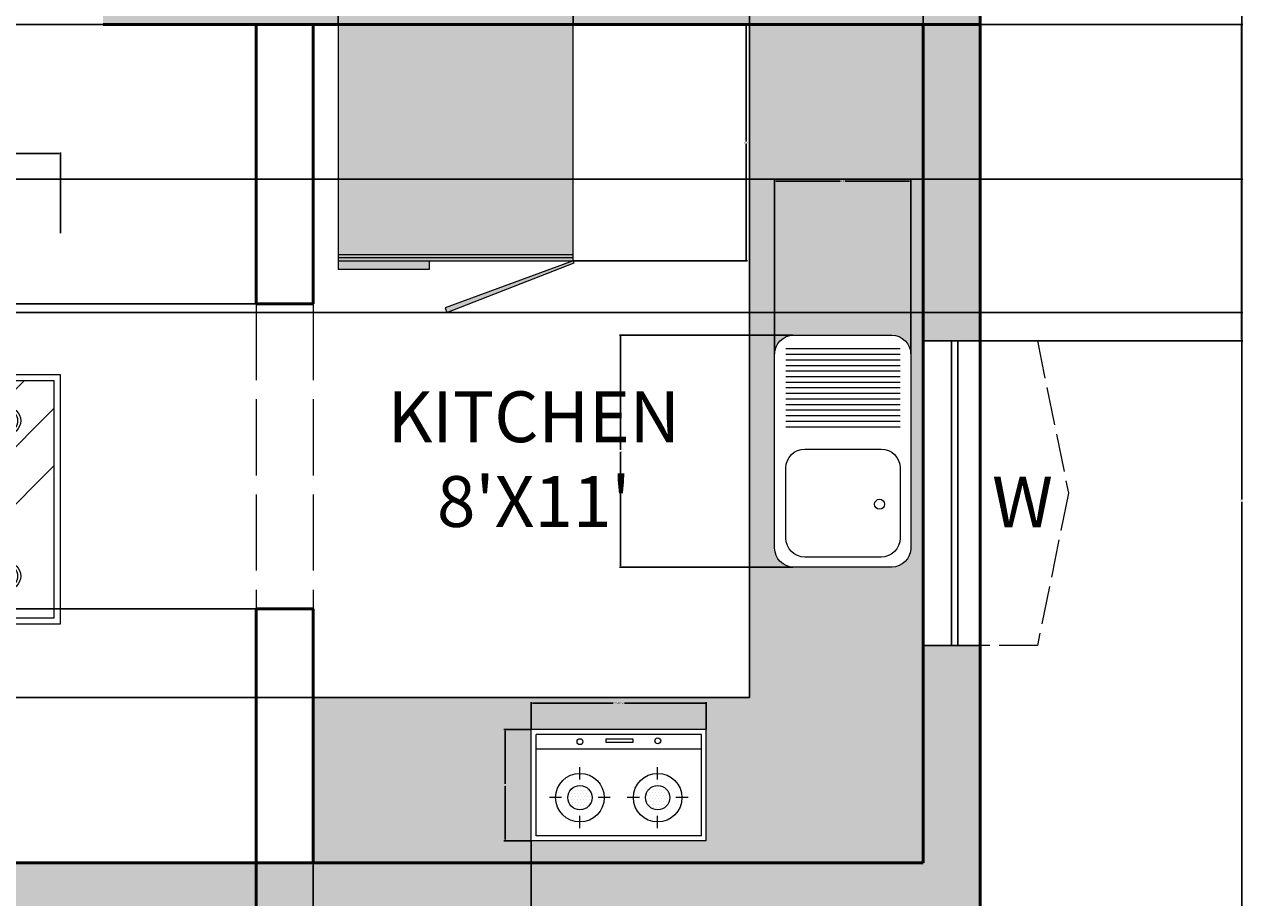
# Model space of a CAD drawing. Units: inches. Extents: x -75 to 416, y -487 to 70.
# Tile 4 of 5: x 224 to 416, y -271 to -133. Entities that reach past the tile are written whole.
import ezdxf

# ---------------------------------------------------------------- set-up
doc = ezdxf.new("R2010")
doc.units = ezdxf.units.IN
doc.header["$MEASUREMENT"] = 0
doc.linetypes.add('ACAD_ISO02W100', pattern=[15, 12, -3])
for name, color, linetype, lineweight in [('A-ANNO-DIMS', 2, 'Continuous', 18), ('A-ANNO-TEXT', 7, 'Continuous', 18), ('A-AREA-IDEN', 7, 'Continuous', 25), ('A-EQPM', 8, 'Continuous', 18), ('A-EQPM-PATT', 252, 'Continuous', 13), ('A-FLOR-CASE', 8, 'Continuous', 25), ('A-FLOR-CASE-PATT', 252, 'Continuous', 13), ('A-FLOR-FIXT', 9, 'Continuous', 18), ('A-FLOR-FIXT-PATT', 9, 'Continuous', 13), ('A-FURN', 8, 'Continuous', 18), ('A-GLAZ', 4, 'Continuous', 25), ('A-GLAZ-OVHD', 4, 'ACAD_ISO02W100', 13), ('A-WALL', 7, 'Continuous', 50), ('A-WALL-OVHD', 7, 'ACAD_ISO02W100', 18), ('A-WALL-PATT', 252, 'Continuous', 13)]:
    doc.layers.add(name, color=color, linetype=linetype, lineweight=lineweight)
doc.styles.get("Standard").update_dxf_attribs({"font": 'arial.ttf'})
doc.dimstyles.get("Standard").update_dxf_attribs({"dimtxt": 0.18, "dimasz": 0.18, "dimexe": 0.18, "dimexo": 0.0625, "dimgap": 0.09, "dimtad": 0, "dimtih": 1, "dimtoh": 1, "dimdec": 4, "dimzin": 0, "dimdsep": 46, "dimtxsty": 'Standard', "dimcen": 0.09, "dimadec": 0, "dimazin": 0, "dimtfac": 1, "dimtdec": 4, "dimtofl": 0, "dimtmove": 0, "dimatfit": 3, "dimfxl": 1, "dimtolj": 1, "dimtzin": 0, "dimarcsym": 0})

# ---------------------------------------------------------------- blocks, each defined once
blk = doc.blocks.new('A$C0FD55737')
for p, q in [((0.2013, 1.6134), (0.1562, 1.3384)), ((0.4912, 1.6302), (0.2211, 1.6302)), ((0.511, 1.6134), (0.5562, 1.3384)), ((0.8828, 1.6134), (0.8376, 1.3384)), ((0.9026, 1.6302), (1.1727, 1.6302)), ((1.1925, 1.6134), (1.2376, 1.3384)), ((0.2362, 1.2584), (0.4762, 1.2584)), ((1.1576, 1.2584), (0.9176, 1.2584)), ((0, 1.2513), (0, 0.4513)), ((1.4, 1.2513), (0, 1.2513)), ((0.02, 1.0725), (0.1788, 1.2313)), ((0.02, 0.7043), (0.547, 1.2313)), ((1.38, 1.2313), (0.02, 1.2313)), ((0.02, 1.2313), (0.02, 0.4713)), ((0.2189, 1.0873), (0.3629, 1.2313)), ((0.3393, 0.4713), (1.0993, 1.2313)), ((0.5234, 0.4713), (1.2834, 1.2313)), ((1.38, 0.4713), (1.38, 1.2313)), ((1.4, 0.4513), (1.4, 1.2513)), ((0.7074, 0.4713), (1.38, 1.1438)), ((0.02, 0.8884), (0.1931, 1.0614)), ((0.8915, 0.4713), (1.38, 0.9597)), ((0.02, 0.4713), (1.38, 0.4713)), ((0, 0.4513), (1.4, 0.4513)), ((0.2362, 0.4371), (0.4762, 0.4371)), ((1.1576, 0.4371), (0.9176, 0.4371)), ((0.2013, 0.0821), (0.1562, 0.3571)), ((0.511, 0.0821), (0.5562, 0.3571)), ((0.8828, 0.0821), (0.8376, 0.3571)), ((1.1925, 0.0821), (1.2376, 0.3571)), ((0.4912, 0.0653), (0.2211, 0.0653)), ((0.9026, 0.0653), (1.1727, 0.0653))]:
    blk.add_line(p, q)
for centre, radius in [((0.1766, 1.1037), 0.0454), ((0.1766, 1.1037), 0.0354), ((1.227, 1.1037), 0.0454), ((1.227, 1.1037), 0.0354), ((0.1766, 0.6052), 0.0454), ((0.1766, 0.6052), 0.0354), ((1.227, 0.6052), 0.0454), ((1.227, 0.6052), 0.0354)]:
    blk.add_circle(centre, radius)
for centre, radius, start, end in [((0.3562, 0.9712), 0.7243, 74.4701, 105.577), ((1.0376, 0.9712), 0.7243, 74.423, 105.5299), ((0.1662, 1.6546), 0.015, 105.4901, 284.2842), ((0.3562, 0.9716), 0.6939, 74.4325, 105.5675), ((0.5461, 1.6546), 0.015, 255.7158, 74.5099), ((0.8477, 1.6546), 0.015, 105.4901, 284.2842), ((1.0376, 0.9716), 0.6939, 74.4325, 105.5675), ((1.2276, 1.6546), 0.015, 255.7158, 74.5099), ((0.2211, 1.6102), 0.02, 90, 170.6717), ((0.4912, 1.6102), 0.02, 9.3283, 90), ((0.9026, 1.6102), 0.02, 90, 170.6717), ((1.1727, 1.6102), 0.02, 9.3283, 90), ((0.2362, 1.3384), 0.08, 180, 270), ((0.4762, 1.3384), 0.08, 270, 0), ((0.9176, 1.3384), 0.08, 180, 270), ((1.1576, 1.3384), 0.08, 270, 0), ((0.2362, 0.3571), 0.08, 90, 180), ((0.4762, 0.3571), 0.08, 0, 90), ((0.9176, 0.3571), 0.08, 90, 180), ((1.1576, 0.3571), 0.08, 0, 90), ((0.2211, 0.0853), 0.02, 189.3283, 270), ((0.4912, 0.0853), 0.02, 270, 350.6717), ((0.9026, 0.0853), 0.02, 189.3283, 270), ((1.1727, 0.0853), 0.02, 270, 350.6717), ((0.1662, 0.0409), 0.015, 75.7158, 254.5099), ((0.3562, 0.7239), 0.6939, 254.4325, 285.5675), ((0.5461, 0.0409), 0.015, 285.4901, 104.2842), ((0.8477, 0.0409), 0.015, 75.7158, 254.5099), ((1.0376, 0.7239), 0.6939, 254.4325, 285.5675), ((1.2276, 0.0409), 0.015, 285.4901, 104.2842), ((0.3562, 0.7243), 0.7243, 254.423, 285.5299), ((1.0376, 0.7243), 0.7243, 254.4701, 285.577)]:
    blk.add_arc(centre, radius, start, end)
blk = doc.blocks.new('A$C475E21CF')
for p, q in [((0, 444.5), (0, 0)), ((0, 444.5), (699.9, 444.5)), ((699.9, 444.5), (699.9, 0)), ((19.4, 425), (19.4, 19.4)), ((19.4, 425), (680.5, 425)), ((194.5, 393.9), (194.5, 345.2)), ((505.4, 393.9), (505.4, 345.2)), ((680.5, 425), (680.5, 19.4)), ((166.9, 300.5), (166.9, 300.5)), ((179.1, 300.5), (179.1, 300.5)), ((185.2, 312.7), (185.2, 312.7)), ((191.2, 300.5), (191.2, 300.5)), ((197.3, 312.7), (197.3, 312.7)), ((203.4, 300.5), (203.4, 300.5)), ((209.5, 312.7), (209.5, 312.7)), ((215.6, 300.5), (215.6, 300.5)), ((227.7, 300.5), (227.7, 300.5)), ((480.2, 304.5), (480.2, 304.5)), ((492.3, 304.5), (492.3, 304.5)), ((498.4, 316.6), (498.4, 316.6)), ((504.5, 304.5), (504.5, 304.5)), ((510.6, 316.6), (510.6, 316.6)), ((516.7, 304.5), (516.7, 304.5)), ((522.7, 316.6), (522.7, 316.6)), ((528.8, 304.5), (528.8, 304.5)), ((541, 304.5), (541, 304.5)), ((72.9, 272.3), (121.6, 272.3)), ((148.7, 264.1), (148.7, 264.1)), ((154.8, 276.2), (154.8, 276.2)), ((154.8, 251.9), (154.8, 251.9)), ((160.9, 288.4), (160.9, 288.4)), ((160.9, 264.1), (160.9, 264.1)), ((166.9, 276.2), (166.9, 276.2)), ((166.9, 251.9), (166.9, 251.9)), ((173, 288.4), (173, 288.4)), ((173, 264.1), (173, 264.1)), ((179.1, 276.2), (179.1, 276.2)), ((179.1, 251.9), (179.1, 251.9)), ((185.2, 288.4), (185.2, 288.4)), ((185.2, 264.1), (185.2, 264.1)), ((191.2, 276.2), (191.2, 276.2)), ((191.2, 251.9), (191.2, 251.9)), ((197.3, 288.4), (197.3, 288.4)), ((197.3, 264.1), (197.3, 264.1)), ((203.4, 276.2), (203.4, 276.2)), ((203.4, 251.9), (203.4, 251.9)), ((209.5, 288.4), (209.5, 288.4)), ((209.5, 264.1), (209.5, 264.1)), ((215.6, 276.2), (215.6, 276.2)), ((215.6, 251.9), (215.6, 251.9)), ((221.6, 288.4), (221.6, 288.4)), ((221.6, 264.1), (221.6, 264.1)), ((227.7, 276.2), (227.7, 276.2)), ((227.7, 251.9), (227.7, 251.9)), ((233.8, 288.4), (233.8, 288.4)), ((233.8, 264.1), (233.8, 264.1)), ((239.9, 276.2), (239.9, 276.2)), ((239.9, 251.9), (239.9, 251.9)), ((267.4, 272.3), (316, 272.3)), ((383.9, 272.3), (432.5, 272.3)), ((462, 268), (462, 268)), ((468, 280.2), (468, 280.2)), ((468, 255.9), (468, 255.9)), ((474.1, 292.3), (474.1, 292.3)), ((474.1, 268), (474.1, 268)), ((480.2, 280.2), (480.2, 280.2)), ((480.2, 255.9), (480.2, 255.9)), ((486.3, 292.3), (486.3, 292.3)), ((486.3, 268), (486.3, 268)), ((492.3, 280.2), (492.3, 280.2)), ((492.3, 255.9), (492.3, 255.9)), ((498.4, 292.3), (498.4, 292.3)), ((498.4, 268), (498.4, 268)), ((504.5, 280.2), (504.5, 280.2)), ((504.5, 255.9), (504.5, 255.9)), ((510.6, 292.3), (510.6, 292.3)), ((510.6, 268), (510.6, 268)), ((516.7, 280.2), (516.7, 280.2)), ((516.7, 255.9), (516.7, 255.9)), ((522.7, 292.3), (522.7, 292.3)), ((522.7, 268), (522.7, 268)), ((528.8, 280.2), (528.8, 280.2)), ((528.8, 255.9), (528.8, 255.9)), ((534.9, 292.3), (534.9, 292.3)), ((534.9, 268), (534.9, 268)), ((541, 280.2), (541, 280.2)), ((541, 255.9), (541, 255.9)), ((547, 292.3), (547, 292.3)), ((547, 268), (547, 268)), ((553.1, 280.2), (553.1, 280.2)), ((553.1, 255.9), (553.1, 255.9)), ((578.4, 272.3), (627, 272.3)), ((160.9, 239.8), (160.9, 239.8)), ((173, 239.8), (173, 239.8)), ((179.1, 227.6), (179.1, 227.6)), ((185.2, 239.8), (185.2, 239.8)), ((191.2, 227.6), (191.2, 227.6)), ((194.5, 199.4), (194.5, 150.8)), ((197.3, 239.8), (197.3, 239.8)), ((203.4, 227.6), (203.4, 227.6)), ((209.5, 239.8), (209.5, 239.8)), ((215.6, 227.6), (215.6, 227.6)), ((221.6, 239.8), (221.6, 239.8)), ((233.8, 239.8), (233.8, 239.8)), ((474.1, 243.7), (474.1, 243.7)), ((486.3, 243.7), (486.3, 243.7)), ((492.3, 231.5), (492.3, 231.5)), ((498.4, 243.7), (498.4, 243.7)), ((504.5, 231.5), (504.5, 231.5)), ((505.4, 199.4), (505.4, 150.8)), ((510.6, 243.7), (510.6, 243.7)), ((516.7, 231.5), (516.7, 231.5)), ((522.7, 243.7), (522.7, 243.7)), ((528.8, 231.5), (528.8, 231.5)), ((534.9, 243.7), (534.9, 243.7)), ((547, 243.7), (547, 243.7)), ((19.4, 77.8), (680.5, 77.8)), ((293.4, 51.9), (400.6, 51.9)), ((293.4, 36.5), (293.4, 51.9)), ((400.6, 51.9), (400.6, 36.5)), ((0, 0), (699.9, 0)), ((19.4, 19.4), (680.5, 19.4)), ((400.6, 36.5), (293.4, 36.5))]:
    blk.add_line(p, q)
for centre, radius in [((194.5, 272.3), 97.2), ((505.4, 272.3), 97.2), ((194.5, 272.3), 48.6), ((505.4, 272.3), 48.6), ((193.9, 45.1), 11.7), ((505.2, 48.5), 11.7)]:
    blk.add_circle(centre, radius)
blk = doc.blocks.new('WIN-48IN')
for p, q in [((0, 9), (0, 0)), ((48, 9), (48, 0)), ((48, 5.5), (0, 5.5)), ((48, 4.5), (0, 4.5))]:
    blk.add_line(p, q)
blk = doc.blocks.new('WIN-SHADE-48IN')
at = {"ltscale": 0.5}
for p, q in [((0, 4.91), (0, 13.91)), ((48, 13.91), (48, 4.91)), ((24, 0), (0, 4.91)), ((48, 4.91), (24, 0))]:
    blk.add_line(p, q, dxfattribs=at)
blk = doc.blocks.new('*D29')
at = {"layer": 'A-ANNO-DIMS', "color": 0, "lineweight": -2, "transparency": 16777216}
for p, q in [((161.08, -166.25), (161.08, -153.53)), ((229.74, -166.25), (229.74, -153.53)), ((161.26, -153.71), (195.2, -153.71)), ((229.56, -153.71), (195.63, -153.71))]:
    blk.add_line(p, q, dxfattribs=at)
at = {"layer": 'A-ANNO-DIMS', "color": 0, "transparency": 16777216}
for points in [[(161.26, -153.68), (161.26, -153.74), (161.08, -153.71)], [(229.56, -153.68), (229.56, -153.74), (229.74, -153.71)]]:
    blk.add_solid(points, dxfattribs=at)
at = {"layer": 'Defpoints', "color": 0, "transparency": 16777216}
for p in [(229.74, -153.71), (161.08, -166.31), (229.74, -166.31)]:
    blk.add_point(p, dxfattribs=at)
at = {"layer": 'A-ANNO-DIMS', "color": 0, "transparency": 16777216, "insert": (195.41, -153.71), "char_height": 0.18, "attachment_point": 5}
blk.add_mtext('\\A1;69', dxfattribs=at)
blk = doc.blocks.new('*D30')
at = {"layer": 'A-ANNO-DIMS', "color": 0, "lineweight": -2, "transparency": 16777216}
for p, q in [((303.87, -244.32), (303.87, -240.07)), ((304.05, -240.25), (316.77, -240.25)), ((331.25, -240.25), (318.53, -240.25)), ((331.43, -244.32), (331.43, -240.07))]:
    blk.add_line(p, q, dxfattribs=at)
at = {"layer": 'A-ANNO-DIMS', "color": 0, "transparency": 16777216}
for points in [[(304.05, -240.22), (304.05, -240.28), (303.87, -240.25)], [(331.25, -240.22), (331.25, -240.28), (331.43, -240.25)]]:
    blk.add_solid(points, dxfattribs=at)
at = {"layer": 'Defpoints', "color": 0, "transparency": 16777216}
for p in [(303.87, -240.25), (303.87, -244.38), (331.43, -244.38)]:
    blk.add_point(p, dxfattribs=at)
at = {"layer": 'A-ANNO-DIMS', "color": 0, "transparency": 16777216, "insert": (317.65, -240.25), "char_height": 0.18, "attachment_point": 5}
blk.add_mtext('\\A1;COOKTOP 28', dxfattribs=at)
blk = doc.blocks.new('*D31')
at = {"layer": 'A-ANNO-DIMS', "color": 0, "lineweight": -2, "transparency": 16777216}
for p, q in [((303.81, -244.38), (299.56, -244.38)), ((299.74, -244.56), (299.74, -252.95)), ((299.74, -261.7), (299.74, -253.31)), ((303.81, -261.88), (299.56, -261.88))]:
    blk.add_line(p, q, dxfattribs=at)
at = {"layer": 'A-ANNO-DIMS', "color": 0, "transparency": 16777216}
for points in [[(299.71, -244.56), (299.77, -244.56), (299.74, -244.38)], [(299.71, -261.7), (299.77, -261.7), (299.74, -261.88)]]:
    blk.add_solid(points, dxfattribs=at)
at = {"layer": 'Defpoints', "color": 0, "transparency": 16777216}
for p in [(303.87, -244.38), (299.74, -261.88), (303.87, -261.88)]:
    blk.add_point(p, dxfattribs=at)
at = {"layer": 'A-ANNO-DIMS', "color": 0, "transparency": 16777216, "insert": (299.74, -253.13), "char_height": 0.18, "attachment_point": 5}
blk.add_mtext('\\A1;17', dxfattribs=at)
blk = doc.blocks.new('*D35')
at = {"layer": 'A-ANNO-DIMS', "color": 0, "lineweight": -2, "transparency": 16777216}
for p, q in [((374.615553, 28.625508), (415.902741, 28.625508)), ((415.722741, 28.445508), (415.722741, -208.194492)), ((415.722741, -445.194492), (415.722741, -208.554492)), ((374.615553, -445.374492), (415.902741, -445.374492))]:
    blk.add_line(p, q, dxfattribs=at)
at = {"layer": 'A-ANNO-DIMS', "color": 0, "transparency": 16777216}
for points in [[(415.692741, 28.445508), (415.752741, 28.445508), (415.722741, 28.625508)], [(415.692741, -445.194492), (415.752741, -445.194492), (415.722741, -445.374492)]]:
    blk.add_solid(points, dxfattribs=at)
at = {"layer": 'Defpoints', "color": 0, "transparency": 16777216}
for p in [(374.553053, 28.625508), (374.553053, -445.374492), (415.722741, -445.374492)]:
    blk.add_point(p, dxfattribs=at)
at = {"layer": 'A-ANNO-DIMS', "color": 0, "transparency": 16777216, "insert": (415.722741, -208.374492), "char_height": 0.18, "attachment_point": 5}
blk.add_mtext('\\A1;474', dxfattribs=at)
blk = doc.blocks.new('*D41')
at = {"layer": 'A-ANNO-DIMS', "color": 0, "lineweight": -2, "transparency": 16777216}
for p, q in [((374.62, -133.37), (415.9, -133.37)), ((415.72, -133.55), (415.72, -158.09)), ((415.72, -182.99), (415.72, -158.45)), ((374.62, -183.17), (415.9, -183.17))]:
    blk.add_line(p, q, dxfattribs=at)
at = {"layer": 'A-ANNO-DIMS', "color": 0, "transparency": 16777216}
for points in [[(415.69, -133.55), (415.75, -133.55), (415.72, -133.37)], [(415.69, -182.99), (415.75, -182.99), (415.72, -183.17)]]:
    blk.add_solid(points, dxfattribs=at)
at = {"layer": 'Defpoints', "color": 0, "transparency": 16777216}
for p in [(374.55, -133.37), (374.55, -183.17), (415.72, -183.17)]:
    blk.add_point(p, dxfattribs=at)
at = {"layer": 'A-ANNO-DIMS', "color": 0, "transparency": 16777216, "insert": (415.72, -158.27), "char_height": 0.18, "attachment_point": 5}
blk.add_mtext('\\A1;49.79', dxfattribs=at)
blk = doc.blocks.new('*D52')
at = {"layer": 'A-ANNO-DIMS', "color": 0, "lineweight": -2, "transparency": 16777216}
for p, q in [((260.49, -133.37), (-74.89, -133.37)), ((-74.71, -133.55), (-74.71, -155.19)), ((-74.71, -177.19), (-74.71, -155.55)), ((260.49, -177.37), (-74.89, -177.37))]:
    blk.add_line(p, q, dxfattribs=at)
at = {"layer": 'A-ANNO-DIMS', "color": 0, "transparency": 16777216}
for points in [[(-74.74, -133.55), (-74.68, -133.55), (-74.71, -133.37)], [(-74.74, -177.19), (-74.68, -177.19), (-74.71, -177.37)]]:
    blk.add_solid(points, dxfattribs=at)
at = {"layer": 'Defpoints', "color": 0, "transparency": 16777216}
for p in [(260.55, -133.37), (-74.71, -177.37), (260.55, -177.37)]:
    blk.add_point(p, dxfattribs=at)
at = {"layer": 'A-ANNO-DIMS', "color": 0, "transparency": 16777216, "insert": (-74.71, -155.37), "char_height": 0.18, "attachment_point": 5}
blk.add_mtext('\\A1;43.99', dxfattribs=at)
blk = doc.blocks.new('*D53')
at = {"layer": 'A-ANNO-DIMS', "color": 0, "lineweight": -2, "transparency": 16777216}
for p, q in [((260.49, -177.37), (-74.89, -177.37)), ((-74.71, -177.55), (-74.71, -201.19)), ((-74.71, -225.19), (-74.71, -201.55)), ((260.49, -225.37), (-74.89, -225.37))]:
    blk.add_line(p, q, dxfattribs=at)
at = {"layer": 'A-ANNO-DIMS', "color": 0, "transparency": 16777216}
for points in [[(-74.74, -177.55), (-74.68, -177.55), (-74.71, -177.37)], [(-74.74, -225.19), (-74.68, -225.19), (-74.71, -225.37)]]:
    blk.add_solid(points, dxfattribs=at)
at = {"layer": 'Defpoints', "color": 0, "transparency": 16777216}
for p in [(260.55, -177.37), (-74.71, -225.37), (260.55, -225.37)]:
    blk.add_point(p, dxfattribs=at)
at = {"layer": 'A-ANNO-DIMS', "color": 0, "transparency": 16777216, "insert": (-74.71, -201.37), "char_height": 0.18, "attachment_point": 5}
blk.add_mtext('\\A1;48', dxfattribs=at)
blk = doc.blocks.new('*D54')
at = {"layer": 'A-ANNO-DIMS', "color": 0, "lineweight": -2, "transparency": 16777216}
for p, q in [((338.22, -133.31), (338.22, 69.98)), ((338.4, 69.8), (351.49, 69.8)), ((365.37, 69.8), (352.28, 69.8)), ((365.55, -133.31), (365.55, 69.98))]:
    blk.add_line(p, q, dxfattribs=at)
at = {"layer": 'A-ANNO-DIMS', "color": 0, "transparency": 16777216}
for points in [[(338.4, 69.83), (338.4, 69.77), (338.22, 69.8)], [(365.37, 69.83), (365.37, 69.77), (365.55, 69.8)]]:
    blk.add_solid(points, dxfattribs=at)
at = {"layer": 'Defpoints', "color": 0, "transparency": 16777216}
for p in [(365.55, 69.8), (338.22, -133.37), (365.55, -133.37)]:
    blk.add_point(p, dxfattribs=at)
at = {"layer": 'A-ANNO-DIMS', "color": 0, "transparency": 16777216, "insert": (351.89, 69.8), "char_height": 0.18, "attachment_point": 5}
blk.add_mtext('\\A1;27.33', dxfattribs=at)
blk = doc.blocks.new('*D55')
at = {"layer": 'A-ANNO-DIMS', "color": 0, "lineweight": -2, "transparency": 16777216}
for p, q in [((269.49, -239.36), (-74.89, -239.36)), ((-74.71, -239.54), (-74.71, -252.19)), ((-74.71, -265.19), (-74.71, -252.55)), ((269.49, -265.37), (-74.89, -265.37))]:
    blk.add_line(p, q, dxfattribs=at)
at = {"layer": 'A-ANNO-DIMS', "color": 0, "transparency": 16777216}
for points in [[(-74.74, -239.54), (-74.68, -239.54), (-74.71, -239.36)], [(-74.74, -265.19), (-74.68, -265.19), (-74.71, -265.37)]]:
    blk.add_solid(points, dxfattribs=at)
at = {"layer": 'Defpoints', "color": 0, "transparency": 16777216}
for p in [(269.55, -239.36), (-74.71, -265.37), (269.55, -265.37)]:
    blk.add_point(p, dxfattribs=at)
at = {"layer": 'A-ANNO-DIMS', "color": 0, "transparency": 16777216, "insert": (-74.71, -252.37), "char_height": 0.18, "attachment_point": 5}
blk.add_mtext('\\A1;26.01', dxfattribs=at)
blk = doc.blocks.new('*D60')
at = {"layer": 'A-ANNO-DIMS', "color": 0, "lineweight": -2, "transparency": 16777216}
for p, q in [((12.62, -157.75), (415.9, -157.75)), ((415.72, -157.93), (415.72, -168.07)), ((415.72, -178.57), (415.72, -168.43)), ((12.62, -178.75), (415.9, -178.75))]:
    blk.add_line(p, q, dxfattribs=at)
at = {"layer": 'A-ANNO-DIMS', "color": 0, "transparency": 16777216}
for points in [[(415.69, -157.93), (415.75, -157.93), (415.72, -157.75)], [(415.69, -178.57), (415.75, -178.57), (415.72, -178.75)]]:
    blk.add_solid(points, dxfattribs=at)
at = {"layer": 'Defpoints', "color": 0, "transparency": 16777216}
for p in [(12.55, -157.75), (12.55, -178.75), (415.72, -178.75)]:
    blk.add_point(p, dxfattribs=at)
at = {"layer": 'A-ANNO-DIMS', "color": 0, "transparency": 16777216, "insert": (415.72, -168.25), "char_height": 0.18, "attachment_point": 5}
blk.add_mtext('\\A1;21', dxfattribs=at)
blk = doc.blocks.new('*D66')
at = {"layer": 'A-ANNO-DIMS', "color": 0, "lineweight": -2, "transparency": 16777216}
for p, q in [((273.46, -133.31), (273.46, 69.98)), ((273.64, 69.8), (291.5, 69.8)), ((310.28, 69.8), (292.43, 69.8)), ((310.46, -133.31), (310.46, 69.98))]:
    blk.add_line(p, q, dxfattribs=at)
at = {"layer": 'A-ANNO-DIMS', "color": 0, "transparency": 16777216}
for points in [[(273.64, 69.83), (273.64, 69.77), (273.46, 69.8)], [(310.28, 69.83), (310.28, 69.77), (310.46, 69.8)]]:
    blk.add_solid(points, dxfattribs=at)
at = {"layer": 'Defpoints', "color": 0, "transparency": 16777216}
for p in [(310.46, 69.8), (273.46, -133.37), (310.46, -133.37)]:
    blk.add_point(p, dxfattribs=at)
at = {"layer": 'A-ANNO-DIMS', "color": 0, "transparency": 16777216, "insert": (291.96, 69.8), "char_height": 0.18, "attachment_point": 5}
blk.add_mtext('\\A1;37.004', dxfattribs=at)
blk = doc.blocks.new('*D67')
at = {"layer": 'A-ANNO-DIMS', "color": 0, "lineweight": -2, "transparency": 16777216}
for p, q in [((310.53, -133.37), (337.9, -133.37)), ((337.72, -133.55), (337.72, -151.81)), ((337.72, -170.43), (337.72, -152.18)), ((310.53, -170.61), (337.9, -170.61))]:
    blk.add_line(p, q, dxfattribs=at)
at = {"layer": 'A-ANNO-DIMS', "color": 0, "transparency": 16777216}
for points in [[(337.69, -133.55), (337.75, -133.55), (337.72, -133.37)], [(337.69, -170.43), (337.75, -170.43), (337.72, -170.61)]]:
    blk.add_solid(points, dxfattribs=at)
at = {"layer": 'Defpoints', "color": 0, "transparency": 16777216}
for p in [(310.46, -133.37), (310.46, -170.61), (337.72, -170.61)]:
    blk.add_point(p, dxfattribs=at)
at = {"layer": 'A-ANNO-DIMS', "color": 0, "transparency": 16777216, "insert": (337.72, -151.99), "char_height": 0.18, "attachment_point": 5}
blk.add_mtext('\\A1;37.24', dxfattribs=at)
blk = doc.blocks.new('*D68')
at = {"layer": 'A-ANNO-DIMS', "color": 0, "lineweight": -2, "transparency": 16777216}
for p, q in [((345.13, -182.29), (317.75, -182.29)), ((317.93, -182.47), (317.93, -200.37)), ((317.93, -218.63), (317.93, -200.73)), ((345.13, -218.81), (317.75, -218.81))]:
    blk.add_line(p, q, dxfattribs=at)
at = {"layer": 'A-ANNO-DIMS', "color": 0, "transparency": 16777216}
for points in [[(317.9, -182.47), (317.96, -182.47), (317.93, -182.29)], [(317.9, -218.63), (317.96, -218.63), (317.93, -218.81)]]:
    blk.add_solid(points, dxfattribs=at)
at = {"layer": 'Defpoints', "color": 0, "transparency": 16777216}
for p in [(317.93, -182.29), (345.19, -182.29), (345.19, -218.81)]:
    blk.add_point(p, dxfattribs=at)
at = {"layer": 'A-ANNO-DIMS', "color": 0, "transparency": 16777216, "insert": (317.93, -200.55), "char_height": 0.18, "attachment_point": 5}
blk.add_mtext('\\A1;36.52', dxfattribs=at)
blk = doc.blocks.new('*D69')
at = {"layer": 'A-ANNO-DIMS', "color": 0, "lineweight": -2, "transparency": 16777216}
for p, q in [((342.19, -185.23), (342.19, -157.85)), ((342.37, -158.03), (352.51, -158.03)), ((363.44, -158.03), (353.3, -158.03)), ((363.62, -185.23), (363.62, -157.85))]:
    blk.add_line(p, q, dxfattribs=at)
at = {"layer": 'A-ANNO-DIMS', "color": 0, "transparency": 16777216}
for points in [[(342.37, -158), (342.37, -158.06), (342.19, -158.03)], [(363.44, -158), (363.44, -158.06), (363.62, -158.03)]]:
    blk.add_solid(points, dxfattribs=at)
at = {"layer": 'Defpoints', "color": 0, "transparency": 16777216}
for p in [(363.62, -158.03), (342.19, -185.29), (363.62, -185.29)]:
    blk.add_point(p, dxfattribs=at)
at = {"layer": 'A-ANNO-DIMS', "color": 0, "transparency": 16777216, "insert": (352.9, -158.03), "char_height": 0.18, "attachment_point": 5}
blk.add_mtext('\\A1;21.43', dxfattribs=at)
blk = doc.blocks.new('*D71')
at = {"layer": 'A-ANNO-DIMS', "color": 0, "lineweight": -2, "transparency": 16777216}
for p, q in [((303.87, -261.95), (303.87, -486.72)), ((269.55, -265.44), (269.55, -486.72)), ((269.73, -486.54), (286.32, -486.54)), ((303.69, -486.54), (287.11, -486.54))]:
    blk.add_line(p, q, dxfattribs=at)
at = {"layer": 'A-ANNO-DIMS', "color": 0, "transparency": 16777216}
for points in [[(269.73, -486.51), (269.73, -486.57), (269.55, -486.54)], [(303.69, -486.51), (303.69, -486.57), (303.87, -486.54)]]:
    blk.add_solid(points, dxfattribs=at)
at = {"layer": 'Defpoints', "color": 0, "transparency": 16777216}
for p in [(303.87, -261.88), (269.55, -265.37), (303.87, -486.54)]:
    blk.add_point(p, dxfattribs=at)
at = {"layer": 'A-ANNO-DIMS', "color": 0, "transparency": 16777216, "insert": (286.71, -486.54), "char_height": 0.18, "attachment_point": 5}
blk.add_mtext('\\A1;34.32', dxfattribs=at)

msp = doc.modelspace()

# ---------------------------------------------------------------- hatches: boundary and pattern name
at = {"layer": 'A-EQPM-PATT'}
h = msp.add_hatch(color=256, dxfattribs=at)
h.dxf.hatch_style = 1
h.set_gradient(color1=(147, 149, 152), color2=(199, 200, 202), tint=1, name='CYLINDER')
h.paths.add_polyline_path([(310.465, -133.3745), (273.461, -133.3745), (273.461, -169.6057), (310.465, -169.6057)])
h.paths.add_polyline_path([(310.465, -169.6057), (273.461, -169.6057), (273.461, -170.0998), (310.465, -170.0998)])
h.paths.add_polyline_path([(310.465, -170.0998), (273.461, -170.0998), (273.461, -170.6149), (310.465, -170.6149)])
h.paths.add_polyline_path([(287.8335, -170.6149), (273.461, -170.6149), (273.461, -171.8852), (287.8335, -171.8852)])
h.paths.add_polyline_path([(310.6449, -170.9123), (310.465, -170.6149), (290.3016, -178.0178), (290.5644, -178.7337)])
at = {"layer": 'A-FLOR-CASE-PATT'}
h = msp.add_hatch(dxfattribs=at)
h.set_pattern_fill('AR-CONC', color=256, scale=0.5)
h.set_pattern_definition([(50, (0, 0), (3.5863, -0.31376), [0.375, -4.125]), (355, (0, 0), (-0.693757, 3.76096), [0.3, -3.3]), (100.45144, (0.299, -0.026), (2.892544, 3.4472), [0.3187, -3.50571]), (46.1842, (0, 1), (5.336207, -0.827596), [0.5625, -6.1875]), (96.6356, (0.4447, 0.931), (4.67331, 4.870593), [0.47805, -5.25857]), (351.1842, (0, 1), (4.67331, 4.87059), [0.45, -4.95]), (21, (0.5, 0.75), (2.984535, -2.013094), [0.375, -4.125]), (326, (0.5, 0.75), (1.216577, 3.62575), [0.3, -3.3]), (71.45144, (0.7487, 0.5822), (4.201112, 1.612656), [0.3187, -3.50571]), (37.5, (0, 0), (0.0607993, 1.6644693), [0, -3.26, 0, -3.35, 0, -3.3125]), (7.5, (0, 0), (1.315348, 1.9720586), [0, -1.91, 0, -3.185, 0, -1.2625]), (327.5, (-1.115, 0), (2.669112, -0.1127744), [0, -1.25, 0, -3.9, 0, -5.175]), (317.5, (-1.615, 0), (2.915931, 0.500525), [0, -1.625, 0, -2.59, 0, -3.675])])
h.paths.add_polyline_path([(365.5531, -133.3745), (338.2223, -133.3745), (338.2223, -239.362), (269.5531, -239.362), (269.5531, -265.3745), (365.5531, -265.3745)])
h.paths.add_polyline_path([(360.6174, -182.2905, -0.41421356), (363.6174, -185.2905), (363.6174, -215.8118, -0.41421356), (360.6174, -218.8118), (345.1886, -218.8118, -0.41421356), (342.1886, -215.8118), (342.1886, -185.2905, -0.41421356), (345.1886, -182.2905)], flags=16)
h.paths.add_polyline_path([(358.9442, -200.2212, -0.41421356), (361.9442, -203.2212), (361.9442, -214.2452, -0.41421356), (358.9442, -217.2452), (346.9581, -217.2452, -0.41421356), (343.9581, -214.2452), (343.9581, -203.2212, -0.41421356), (346.9581, -200.2212)], flags=0)
h.paths.add_polyline_path([(359.4917, -208.9083, -1), (357.9194, -208.9083, -1)], flags=0)
h.paths.add_polyline_path([(331.4284, -244.3832), (331.4284, -261.883), (303.8724, -261.883), (303.8724, -244.3832)], flags=16)
h.paths.add_polyline_path([(330.6628, -245.1489), (330.6628, -261.1173), (304.6381, -261.1173), (304.6381, -245.1489)], flags=0)
h.paths.add_polyline_path([(324.2526, -246.1573, -1), (323.3338, -246.1573, -1)], flags=0)
h.paths.add_polyline_path([(319.8771, -245.8199), (319.8771, -246.4272), (315.6559, -246.4272), (315.6559, -245.8199)], flags=0)
h.paths.add_polyline_path([(327.6001, -255.1039, -1), (319.9433, -255.1039, -1)], flags=0)
h.paths.add_polyline_path([(311.9966, -246.2922, -1), (311.0778, -246.2922, -1)], flags=0)
h.paths.add_polyline_path([(325.6859, -255.1039, -1), (321.8575, -255.1039, -1)], flags=0)
h.paths.add_polyline_path([(315.3575, -255.1039, -1), (307.7007, -255.1039, -1)], flags=0)
h.paths.add_polyline_path([(313.4433, -255.1039, -1), (309.6149, -255.1039, -1)], flags=0)
at = {"layer": 'A-FLOR-FIXT-PATT'}
h = msp.add_hatch(dxfattribs=at)
h.set_pattern_fill('ANSI31', color=256, scale=7.02528, angle=-45, style=0)
h.paths.add_polyline_path([(343.9581, -196.7913), (361.9442, -196.7913), (361.9442, -183.6188), (343.9581, -183.6188)])
at = {"layer": 'A-WALL-PATT'}
h = msp.add_hatch(color=256, dxfattribs=at)
h.dxf.hatch_style = 1
h.paths.add_polyline_path([(84.8603, 28.6255), (3.5531, 28.6255), (3.5531, -23.8141), (12.5531, -23.8141), (12.5531, 19.6255), (84.8603, 19.6255)])
h.paths.add_polyline_path([(263.7442, 28.6255), (132.8603, 28.6255), (132.8603, 19.6255), (146.5531, 19.6255), (180.5531, 19.6255), (180.5531, -124.3745), (180.5531, -133.3745), (200.467, -133.3745), (200.467, -124.3745), (189.5531, -124.3745), (189.5531, 19.6255), (263.7442, 19.6255)])
h.paths.add_polyline_path([(374.5531, 28.6255), (311.7442, 28.6255), (311.7442, 19.6255), (327.5531, 19.6255), (365.5531, 19.6255), (365.5531, -37.0191), (374.5531, -37.0191)])
h.paths.add_polyline_path([(144.5531, -124.3745), (12.5531, -124.3745), (12.5531, -71.8141), (3.5531, -71.8141), (3.5531, -148.6403), (12.5531, -148.6403), (12.5531, -133.3745), (144.5531, -133.3745)])
h.paths.add_polyline_path([(117.5531, -133.3745), (108.5531, -133.3745), (108.5531, -161.7866), (117.5531, -161.7866)])
h.paths.add_polyline_path([(374.5531, -85.0191), (365.5531, -85.0191), (365.5531, -124.3745), (236.467, -124.3745), (236.467, -133.3745), (374.5531, -133.3745)])
h.paths.add_polyline_path([(374.5531, -133.3745), (365.5531, -133.3745), (365.5531, -183.1692), (374.5531, -183.1692)])
h.paths.add_polyline_path([(374.5531, -231.1692), (365.5531, -231.1692), (365.5531, -265.3745), (260.5531, -265.3745), (260.5531, -274.3745), (374.5531, -274.3745)])
h.paths.add_polyline_path([(260.5531, -265.3745), (215.5531, -265.3745), (215.5531, -288.4908), (224.5531, -288.4908), (224.5531, -274.3745), (260.5531, -274.3745)])
h.paths.add_polyline_path([(374.5531, -274.3745), (365.5531, -274.3745), (365.5531, -345.9302), (374.5531, -345.9302)])
h.paths.add_polyline_path([(374.5531, -393.9302), (365.5531, -393.9302), (365.5531, -436.3745), (321.1982, -436.3745), (321.1982, -445.3745), (374.5531, -445.3745)])
h.paths.add_polyline_path([(224.5531, -324.4908), (215.5531, -324.4908), (215.5531, -445.3745), (273.1982, -445.3745), (273.1982, -436.3745), (265.0531, -436.3745), (245.0531, -436.3745), (224.5531, -436.3745)])
h.paths.add_polyline_path([(12.5531, -183.233), (3.5531, -183.233), (3.5531, -214.3745), (117.5531, -214.3745), (117.5531, -197.7866), (108.5531, -197.7866), (108.5531, -205.3745), (12.5531, -205.3745)])
h.paths.add_polyline_path([(12.5531, -214.3745), (3.5531, -214.3745), (3.5531, -290.2477), (12.5531, -290.2477)])
h.paths.add_polyline_path([(75.0426, -381.3745), (12.5531, -381.3745), (12.5531, -350.2477), (3.5531, -350.2477), (3.5531, -390.3745), (75.0426, -390.3745)])
h.paths.add_polyline_path([(154.4537, -381.3745), (123.0426, -381.3745), (123.0426, -390.3745), (154.4537, -390.3745)])
h.paths.add_polyline_path([(215.5531, -381.3745), (202.4537, -381.3745), (202.4537, -390.3745), (215.5531, -390.3745)])

# ---------------------------------------------------------------- linework, layer by layer
at = {"layer": 'A-EQPM'}
for p, q in [((273.461, -133.3745), (273.461, -170.6149)), ((310.465, -170.6149), (310.465, -133.3745)), ((273.461, -169.6057), (310.465, -169.6057)), ((310.465, -170.0998), (273.461, -170.0998)), ((273.461, -170.6149), (310.465, -170.6149)), ((273.461, -170.6149), (273.461, -171.8852)), ((287.8335, -171.8852), (287.8335, -170.6149)), ((310.465, -170.6149), (290.3016, -178.0178)), ((310.6449, -170.9123), (310.465, -170.6149)), ((273.461, -171.8852), (287.8335, -171.8852)), ((290.5644, -178.7337), (310.6449, -170.9123)), ((290.3016, -178.0178), (290.5644, -178.7337))]:
    msp.add_line(p, q, dxfattribs=at)
at = {"layer": 'A-FLOR-CASE'}
for p, q in [((338.2223, -133.3745), (338.2223, -239.362)), ((338.2223, -239.362), (269.5531, -239.362))]:
    msp.add_line(p, q, dxfattribs=at)
at = {"layer": 'A-FLOR-FIXT'}
for points in [[(345.1886, -182.2905), (360.6174, -182.2905, -0.41421356), (363.6174, -185.2905), (363.6174, -215.8118, -0.41421356), (360.6174, -218.8118), (345.1886, -218.8118, -0.41421356), (342.1886, -215.8118), (342.1886, -185.2905, -0.41421356)], [(346.9581, -200.2212), (358.9442, -200.2212, -0.41421356), (361.9442, -203.2212), (361.9442, -214.2452, -0.41421356), (358.9442, -217.2452), (346.9581, -217.2452, -0.41421356), (343.9581, -214.2452), (343.9581, -203.2212, -0.41421356)]]:
    msp.add_lwpolyline(points, format="xyb", close=True, dxfattribs=at)
msp.add_circle((358.7055, -208.9083), 0.7862, dxfattribs=at)
at = {"layer": 'A-WALL'}
for p, q in [((374.5531, 28.6255), (374.5531, -445.3745)), ((236.467, -133.3745), (374.5531, -133.3745)), ((260.5531, -133.3745), (260.5531, -177.367)), ((269.5531, -133.3745), (269.5531, -177.367)), ((365.5531, -133.3745), (365.5531, -265.3745)), ((260.5531, -177.367), (269.5531, -177.367)), ((260.5531, -225.367), (269.5531, -225.367)), ((260.5531, -225.367), (260.5531, -274.3745)), ((269.5531, -225.367), (269.5531, -265.3745)), ((215.5531, -265.3745), (365.5531, -265.3745))]:
    msp.add_line(p, q, dxfattribs=at)
at = {"layer": 'A-WALL-OVHD'}
for p, q in [((260.5531, -177.367), (260.5531, -225.367)), ((269.5531, -177.367), (269.5531, -225.367))]:
    msp.add_line(p, q, dxfattribs=at)

# ---------------------------------------------------------------- block references
at = {"layer": 'A-EQPM', "xscale": 0.0393700787401575, "yscale": 0.0393700787401575, "zscale": 0.0393700787401575, "rotation": 180}
msp.add_blockref('A$C475E21CF', (331.4284, -244.3832), dxfattribs=at)
at = {"layer": 'A-FURN', "xscale": 49.04285923157839, "yscale": 49.04285923157839, "zscale": 49.04285923157839}
msp.add_blockref('A$C0FD55737', (161.0849, -249.899), dxfattribs=at)
at = {"layer": 'A-GLAZ', "rotation": 270.0000000000002}
msp.add_blockref('WIN-48IN', (365.5535, -183.1696), dxfattribs=at)
at = {"layer": 'A-GLAZ-OVHD', "rotation": 89.99999999999984}
msp.add_blockref('WIN-SHADE-48IN', (388.4626, -231.1694), dxfattribs=at)

# ---------------------------------------------------------------- texts
at = {"layer": 'A-ANNO-TEXT', "insert": (373.6515, -204.5599), "char_height": 8, "attachment_point": 1}
msp.add_mtext_dynamic_manual_height_columns('\\pxqc;W', width=15.130285, gutter_width=1, heights=[0], dxfattribs=at)
at = {"layer": 'A-AREA-IDEN', "insert": (232.0892, -191.1469), "char_height": 8, "attachment_point": 1}
msp.add_mtext_dynamic_manual_height_columns("\\pxqc;KITCHEN\\P8'X11'", width=144.357858, gutter_width=1, heights=[0], dxfattribs=at)

# ---------------------------------------------------------------- dimensions: what is measured, and where the dimension line sits
at = {"layer": 'A-ANNO-DIMS'}
for base, p1, p2, override, picture, middle in [((310.465, 69.7952), (273.461, -133.3745), (310.465, -133.3745), {"dimdec": 3, "dimlfac": 1, "dimrnd": 0, "dimzin": 0, "dimdsep": 46, "dimlunit": 2}, '*D66', (291.963, 69.7952)), ((365.5531, 69.7952), (338.2223, -133.3745), (365.5531, -133.3745), {"dimdec": 2, "dimlfac": 1, "dimrnd": 0, "dimzin": 0, "dimdsep": 46, "dimlunit": 2}, '*D54', (351.8877, 69.7952)), ((229.745, -153.7078), (161.085, -166.3112), (229.745, -166.3112), {"dimdec": 0, "dimlfac": 1, "dimrnd": 0, "dimzin": 0, "dimdsep": 46, "dimlunit": 2}, '*D29', (195.415, -153.7078)), ((363.6174, -158.0305), (342.1886, -185.2905), (363.6174, -185.2905), {"dimdec": 2, "dimlfac": 1, "dimrnd": 0, "dimzin": 0, "dimdsep": 46, "dimlunit": 2}, '*D69', (352.903, -158.0305)), ((303.8724, -486.5442), (269.5531, -265.3745), (303.8724, -261.883), {"dimdec": 2, "dimlfac": 1, "dimrnd": 0, "dimzin": 0, "dimdsep": 46, "dimlunit": 2}, '*D71', (286.7127, -486.5442))]:
    dim = msp.add_linear_dim(base=base, p1=p1, p2=p2, dimstyle='Standard', override=override, dxfattribs=at)
    dim.commit()
    dim.dimension.update_dxf_attribs({"geometry": picture, "text_midpoint": middle})
for base, p1, p2, angle, override, picture, middle in [((415.7227, -445.3745), (374.5531, 28.6255), (374.5531, -445.3745), 90, {"dimdec": 0, "dimlfac": 1, "dimrnd": 0, "dimzin": 0, "dimdsep": 46, "dimlunit": 2}, '*D35', (415.7227, -208.3745)), ((-74.7069, -177.367), (260.5531, -133.3745), (260.5531, -177.367), 90, {"dimdec": 2, "dimlfac": 1, "dimrnd": 0, "dimzin": 0, "dimdsep": 46, "dimlunit": 2}, '*D52', (-74.7069, -155.3707)), ((337.725, -170.6149), (310.465, -133.3745), (310.465, -170.6149), 270, {"dimdec": 2, "dimlfac": 1, "dimrnd": 0, "dimzin": 0, "dimdsep": 46, "dimlunit": 2}, '*D67', (337.725, -151.9947)), ((415.7227, -183.1692), (374.5531, -133.3745), (374.5531, -183.1692), 90, {"dimdec": 2, "dimlfac": 1, "dimrnd": 0, "dimzin": 0, "dimdsep": 46, "dimlunit": 2}, '*D41', (415.7227, -158.2718)), ((415.7227, -178.7524), (12.5531, -157.7524), (12.5531, -178.7524), 90, {"dimdec": 0, "dimlfac": 1, "dimrnd": 0, "dimzin": 0, "dimdsep": 46, "dimlunit": 2}, '*D60', (415.7227, -168.2524)), ((-74.7069, -225.367), (260.5531, -177.367), (260.5531, -225.367), 90, {"dimdec": 0, "dimlfac": 1, "dimrnd": 0, "dimzin": 0, "dimdsep": 46, "dimlunit": 2}, '*D53', (-74.7069, -201.367)), ((317.9286, -182.2905), (345.1886, -218.8118), (345.1886, -182.2905), 90, {"dimdec": 2, "dimlfac": 1, "dimrnd": 0, "dimzin": 0, "dimdsep": 46, "dimlunit": 2}, '*D68', (317.9286, -200.5511)), ((-74.7069, -265.3745), (269.5531, -239.362), (269.5531, -265.3745), 90, {"dimdec": 2, "dimlfac": 1, "dimrnd": 0, "dimzin": 0, "dimdsep": 46, "dimlunit": 2}, '*D55', (-74.7069, -252.3682)), ((299.739, -261.883), (303.8724, -244.3832), (303.8724, -261.883), 270, {"dimdec": 0, "dimlfac": 1, "dimrnd": 0, "dimzin": 0, "dimdsep": 46, "dimlunit": 2}, '*D31', (299.739, -253.1331))]:
    dim = msp.add_linear_dim(base=base, p1=p1, p2=p2, angle=angle, dimstyle='Standard', override=override, dxfattribs=at)
    dim.commit()
    dim.dimension.update_dxf_attribs({"geometry": picture, "text_midpoint": middle})
dim = msp.add_linear_dim(base=(303.8724, -240.2498), p1=(331.4284, -244.3832), p2=(303.8724, -244.3832), angle=180, text='COOKTOP <>', dimstyle='Standard', override={"dimdec": 0, "dimlfac": 1, "dimrnd": 0, "dimzin": 0, "dimdsep": 46, "dimlunit": 2}, dxfattribs=at)
dim.commit()
dim.dimension.update_dxf_attribs({"geometry": '*D30', "text_midpoint": (317.6504, -240.2498)})

doc.saveas('drawing.dxf')
